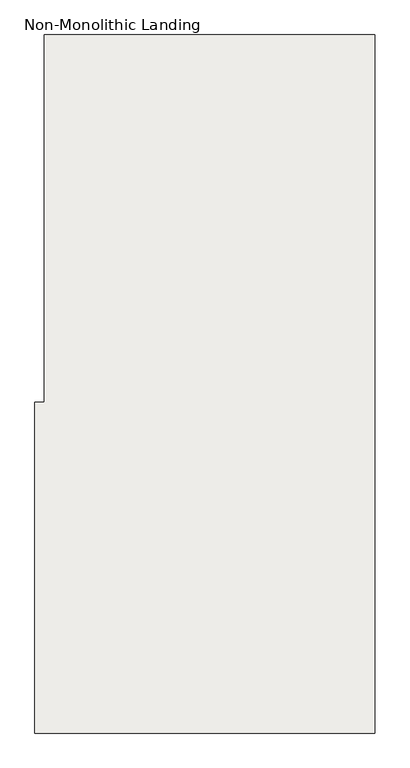
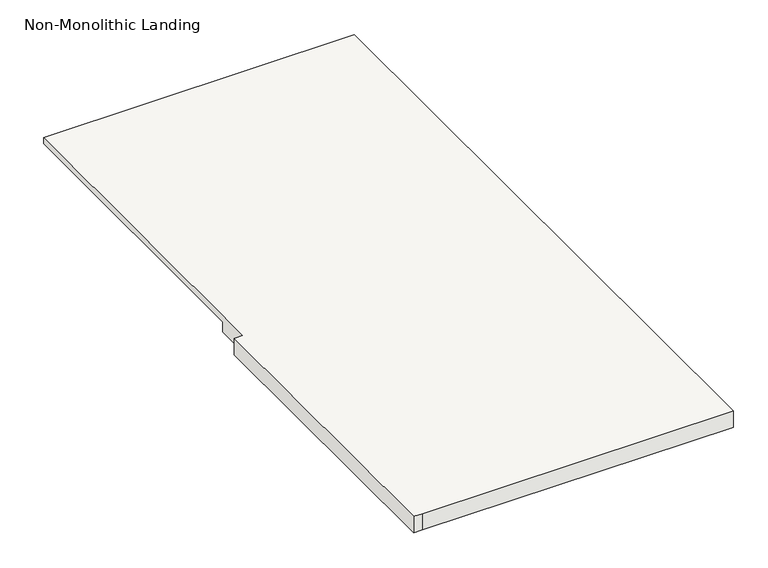
"""IFC4 building model written with IfcOpenShell, lengths in millimetres: slab geometry, Non-Monolithic Landing."""

from ifc_helpers import new_model, si_unit, origin, place, context, project, spatial, faceted_brep, source, transform, mapped, element, save


def non_monolithic_landing_9ec975f3(model_context):
    return source(origin(), model_context, "Body", "Brep", [
        faceted_brep([(923.4845537, -3822.9544725, 11182.35), (948.8845537, -3822.9544725, 11156.95), (948.8845537, -4737.3544725, 11156.95), (923.4845537, -4737.3544725, 11182.35), (923.4845537, -4838.9544725, 11201.4), (898.0845537, -4838.9544725, 11201.4), (898.0845537, -5753.3544725, 11201.4), (923.4845537, -5753.3544725, 11201.4), (1837.8845537, -5753.3544725, 11201.4), (1837.8845537, -3822.9544725, 11201.4), (923.4845537, -3822.9544725, 11201.4), (948.8845537, -4737.3544725, 11150.6), (948.8845537, -3822.9544725, 11150.6), (1837.8845537, -3822.9544725, 11150.6), (1837.8845537, -5753.3544725, 11150.6), (923.4845537, -5753.3544725, 11150.6), (898.0845537, -5753.3544725, 11150.6), (898.0845537, -4838.9544725, 11150.6), (923.4845537, -4838.9544725, 11150.6), (923.4845537, -4737.3544725, 11150.6)], [[[0, 1, 2, 3]], [[4, 5, 6, 7, 8, 9, 10]], [[11, 12, 13, 14, 15, 16, 17, 18, 19]], [[12, 11, 2, 1]], [[11, 19, 3, 2]], [[4, 10, 0, 3, 19, 18]], [[5, 4, 18, 17]], [[6, 5, 17, 16]], [[7, 6, 16, 15]], [[8, 7, 15, 14]], [[9, 8, 14, 13]], [[10, 9, 13, 12, 1, 0]]]),
    ])


if __name__ == "__main__":
    model = new_model("IFC4")
    model_context = context("Model", 3, world=origin())
    ifc_project = project(units=[si_unit("LENGTHUNIT", "METRE", prefix="MILLI")], contexts=[model_context])
    site = spatial("IfcSite", under=ifc_project)
    building = spatial("IfcBuilding", under=site)
    placement = place(None, origin())
    non_monolithic_landing_shape = non_monolithic_landing_9ec975f3(model_context)
    element("IfcSlab", 1, ObjectType="Non-Monolithic Landing", at=placement, inside=building, context=model_context, shape_type="MappedRepresentation", body=[
        mapped(non_monolithic_landing_shape, transform((0.0, 0.0, 0.0), x_axis=(1.0, 0.0, 0.0), y_axis=(0.0, 1.0, 0.0), z_axis=(0.0, 0.0, 1.0))),
    ])
    save(model, "model.ifc")
